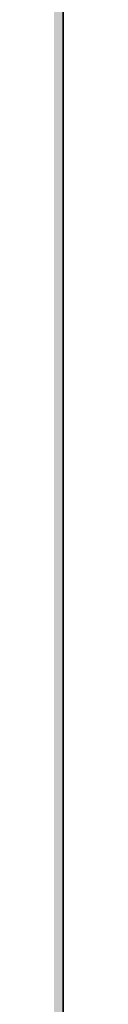
# Model space of a CAD drawing. Units: inches. Extents: x 2083 to 3317, y 1141 to 2115.
# Tile 176 of 256: x 3126.95976 to 3126.95983, y 1263.27402 to 1263.29018. Entities that reach past the tile are written whole.
import ezdxf

# ---------------------------------------------------------------- set-up
doc = ezdxf.new("R2010")
doc.units = ezdxf.units.IN
doc.layers.add('A-ANNO-DIMS', color=2, linetype='Continuous', lineweight=18)
doc.layers.add('A-WALL', color=7, linetype='Continuous', lineweight=35)
doc.layers.add('A-WALL-PATT', color=251, linetype='Continuous', lineweight=13, true_color=0x636466)
doc.styles.get("Standard").update_dxf_attribs({"font": 'arial.ttf'})
doc.dimstyles.new('ISO-25', dxfattribs={"dimtxt": 12, "dimasz": 12, "dimexe": 1.25, "dimexo": 0.625, "dimtad": 1, "dimlunit": 3, "dimtxsty": 'Standard', "dimcen": 2.5, "dimadec": 0, "dimazin": 0, "dimtfac": 1, "dimtmove": 0, "dimatfit": 3, "dimfxl": 1, "dimarcsym": 0})

# ---------------------------------------------------------------- blocks, each defined once
blk = doc.blocks.new('*D9')
at = {"layer": 'A-ANNO-DIMS', "color": 0, "lineweight": -2, "transparency": 16777216}
for p, q in [((3127.584783, 1486.76136), (3190.40309, 1486.76136)), ((3189.15309, 1474.76136), (3189.15309, 1275.26136)), ((3127.584783, 1263.26136), (3190.40309, 1263.26136))]:
    blk.add_line(p, q, dxfattribs=at)
at = {"layer": 'A-ANNO-DIMS', "color": 0, "transparency": 16777216}
for points in [[(3187.15309, 1474.76136), (3191.15309, 1474.76136), (3189.15309, 1486.76136)], [(3187.15309, 1275.26136), (3191.15309, 1275.26136), (3189.15309, 1263.26136)]]:
    blk.add_solid(points, dxfattribs=at)
at = {"layer": 'Defpoints', "color": 0, "transparency": 16777216}
for p in [(3126.959783, 1486.76136), (3126.959783, 1263.26136), (3189.15309, 1263.26136)]:
    blk.add_point(p, dxfattribs=at)
at = {"layer": 'A-ANNO-DIMS', "color": 0, "transparency": 16777216, "insert": (3182.401214, 1375.01136), "char_height": 12, "attachment_point": 5, "rotation": 90}
blk.add_mtext('18\'-7.5"', dxfattribs=at)
blk = doc.blocks.new('*D26')
at = {"layer": 'A-ANNO-DIMS', "color": 0, "lineweight": -2, "transparency": 16777216}
for p, q in [((3088.985844, 1274.915092), (3088.985844, 1270.951963)), ((3111.240037, 1274.915092), (3111.240037, 1270.951963)), ((3076.985844, 1272.201963), (2840.262447, 1272.201963)), ((3111.240037, 1272.201963), (3088.985844, 1272.201963)), ((3123.240037, 1272.201963), (3135.240037, 1272.201963))]:
    blk.add_line(p, q, dxfattribs=at)
at = {"layer": 'A-ANNO-DIMS', "color": 0, "transparency": 16777216}
for points in [[(3076.985844, 1274.201963), (3076.985844, 1270.201963), (3088.985844, 1272.201963)], [(3123.240037, 1274.201963), (3123.240037, 1270.201963), (3111.240037, 1272.201963)]]:
    blk.add_solid(points, dxfattribs=at)
at = {"layer": 'Defpoints', "color": 0, "transparency": 16777216}
for p in [(3088.985844, 1275.540092), (3111.240037, 1275.540092), (3088.985844, 1272.201963)]:
    blk.add_point(p, dxfattribs=at)
at = {"layer": 'A-ANNO-DIMS', "color": 0, "transparency": 16777216, "insert": (2952.624146, 1279.031602), "char_height": 12, "attachment_point": 5}
blk.add_mtext('NIGHTSTAND 1\'-10 1/2" TYP.', dxfattribs=at)
blk = doc.blocks.new('*D27')
at = {"layer": 'A-ANNO-DIMS', "color": 0, "lineweight": -2, "transparency": 16777216}
for p, q in [((3114.578165, 1309.794285), (3114.578165, 1321.794285)), ((3111.865037, 1297.794285), (3115.828165, 1297.794285)), ((3114.578165, 1297.794285), (3114.578165, 1275.540092)), ((3111.865037, 1275.540092), (3115.828165, 1275.540092)), ((3114.578165, 1263.540092), (3114.578165, 1140.988591))]:
    blk.add_line(p, q, dxfattribs=at)
at = {"layer": 'A-ANNO-DIMS', "color": 0, "transparency": 16777216}
for points in [[(3112.578165, 1309.794285), (3116.578165, 1309.794285), (3114.578165, 1297.794285)], [(3112.578165, 1263.540092), (3116.578165, 1263.540092), (3114.578165, 1275.540092)]]:
    blk.add_solid(points, dxfattribs=at)
at = {"layer": 'Defpoints', "color": 0, "transparency": 16777216}
for p in [(3111.240037, 1297.794285), (3111.240037, 1275.540092), (3114.578165, 1275.540092)]:
    blk.add_point(p, dxfattribs=at)
at = {"layer": 'A-ANNO-DIMS', "color": 0, "transparency": 16777216, "insert": (3107.748527, 1196.264342), "char_height": 12, "attachment_point": 5, "rotation": 90}
blk.add_mtext('1\'-10 1/2" TYP.', dxfattribs=at)

msp = doc.modelspace()

# ---------------------------------------------------------------- hatches: boundary and pattern name
at = {"layer": 'A-WALL-PATT'}
h = msp.add_hatch(color=256, dxfattribs=at)
h.dxf.hatch_style = 1
h.paths.add_polyline_path([(3126.959783, 2020.76136), (2748.959783, 2020.76136), (2604.959783, 2020.76136), (2226.959783, 2020.76136), (2226.959783, 1702.76136), (2466.959783, 1702.76136), (2466.959783, 1582.76136), (2418.959783, 1582.76136), (2418.959783, 1477.76136), (2226.959783, 1477.76136), (2226.959783, 1263.26136), (2544.959783, 1263.26136), (2544.959783, 1411.76136), (2604.959783, 1411.76136), (2685.959783, 1411.76136), (2685.959783, 1420.76136), (2604.959783, 1420.76136), (2604.959783, 1573.76136), (2604.959783, 1702.76136), (2604.959783, 2011.76136), (2748.959783, 2011.76136), (2748.959783, 1702.76136), (2862.959783, 1702.76136), (2862.959783, 1621.76136), (2871.959783, 1621.76136), (2871.959783, 1702.76136), (2883.959783, 1702.76136), (2883.959783, 1706.939459, -0.026459), (2883.959783, 1711.76136), (2757.959783, 1711.76136), (2757.959783, 1807.76136), (2787.959783, 1807.76136), (2787.959783, 1812.26136), (2757.959783, 1812.26136), (2757.959783, 2011.76136), (2877.959783, 2011.76136), (2877.959783, 1812.26136), (2847.959783, 1812.26136), (2847.959783, 1807.76136), (2889.835742, 1807.76136), (2889.835742, 1812.26136), (2882.459783, 1812.26136), (2882.459783, 2011.76136), (3117.959783, 2011.76136), (3117.959783, 1812.26136), (2937.835742, 1812.26136), (2937.835742, 1807.76136), (2995.709783, 1807.76136), (2995.709783, 1796.117666), (3000.209783, 1796.117666), (3000.209783, 1807.76136), (3117.959783, 1807.76136), (3117.959783, 1711.76136), (3000.209783, 1711.76136), (3000.209783, 1760.117666), (2998.572705, 1760.117666, -0.020711), (2995.709783, 1760.117666), (2995.709783, 1711.76136), (2931.959783, 1711.76136), (2931.959783, 1702.76136), (3126.959783, 1702.76136)])
h.paths.add_polyline_path([(2471.459783, 2011.76136), (2471.459783, 1810.01136), (2462.716936, 1810.01136), (2462.716936, 1805.51136), (2505.959783, 1805.51136), (2505.959783, 1810.01136), (2475.959783, 1810.01136), (2475.959783, 2011.76136), (2595.959783, 2011.76136), (2595.959783, 1810.01136), (2565.959783, 1810.01136), (2565.959783, 1805.51136), (2595.959783, 1805.51136), (2595.959783, 1711.76136), (2235.959783, 1711.76136), (2235.959783, 1805.51136), (2353.709783, 1805.51136), (2353.709783, 1796.054162), (2358.209783, 1796.054162), (2358.209783, 1805.51136), (2414.716936, 1805.51136), (2414.716936, 1810.01136), (2235.959783, 1810.01136), (2235.959783, 2011.76136)], flags=16)
h.paths.add_polyline_path([(2270.204734, 1994.610008), (2270.204734, 1970.610008), (2246.204734, 1970.610008), (2246.204734, 1994.610008)], flags=0)
edge = h.paths.add_edge_path(flags=0)
edge.add_ellipse((2332.027391, 1899.798176), major_axis=(-3.042994, 3.042994), ratio=0.16825245, start_angle=-161.332166, end_angle=-156.307114, ccw=False)
edge.add_ellipse((2333.082037, 1898.74353), major_axis=(-1.054646, 1.054646), ratio=0.4535321, start_angle=-123.371019, end_angle=-94.159107)
edge = h.paths.add_edge_path(flags=0)
edge.add_ellipse((2332.027391, 1968.87629), major_axis=(3.042994, 3.042994), ratio=0.16825245, start_angle=18.667834, end_angle=23.692886)
edge.add_spline(control_points=[(2332.925596, 1970.691105), (2332.226768, 1970.3361), (2330.893709, 1969.658905), (2328.41308, 1970.932138), (2327.203934, 1967.748712), (2324.709596, 1969.955589), (2322.532822, 1967.012354), (2320.012846, 1971.295812), (2317.680308, 1968.157845), (2316.040526, 1967.102047), (2315.426904, 1966.809602)], knot_values=[0, 0, 0, 0, 2.267059, 4.324559, 6.685584, 8.878641, 11.121502, 14.300359, 17.755284, 19.732645, 19.732645, 19.732645, 19.732645], degree=3, periodic=0)
edge.add_ellipse((2332.027391, 1968.87629), major_axis=(3.042994, 3.042994), ratio=0.16825245, start_angle=18.667834, end_angle=23.692886, ccw=False)
edge.add_ellipse((2333.082037, 1969.930936), major_axis=(1.054646, 1.054646), ratio=0.4535321, start_angle=56.628981, end_angle=85.840893, ccw=False)
edge = h.paths.add_edge_path(flags=0)
edge.add_spline(control_points=[(2296.428287, 1967.987908), (2293.627804, 1965.336314), (2287.703624, 1959.727094), (2299.74386, 1949.995699), (2294.532591, 1935.668528), (2290.573228, 1920.603512), (2293.394124, 1909.973691), (2296.185407, 1904.966543)], knot_values=[0.099185, 0.099185, 0.099185, 0.099185, 0.345301, 0.619822, 0.982653, 1.386093, 1.810555, 1.810555, 1.810555, 1.810555], degree=3, periodic=0)
edge.add_spline(control_points=[(2296.185407, 1904.966543), (2297.383582, 1902.6193), (2298.000969, 1901.949312), (2298.55297, 1901.468155)], knot_values=[0.006246, 0.006246, 0.006246, 0.006246, 0.055476, 0.055476, 0.055476, 0.055476], degree=3, periodic=0)
edge.add_spline(control_points=[(2298.55297, 1901.468155), (2297.258612, 1900.923224), (2295.225294, 1900.232126), (2293.060229, 1900.614205), (2292.101423, 1900.788415), (2292.089578, 1900.790568)], knot_values=[0.312835, 0.312835, 0.312835, 0.312835, 0.40178, 0.474987, 0.475903, 0.475903, 0.475903, 0.475903], degree=3, periodic=0)
edge.add_arc((2292.793646, 1904.664109), 3.937008, 215.420897, 259.698179, ccw=False)
edge.add_spline(control_points=[(2289.585314, 1902.382304), (2289.476652, 1902.535087), (2289.36848, 1902.688035), (2289.260865, 1902.84117)], knot_values=[0.102872, 0.102872, 0.102872, 0.102872, 0.116896, 0.116896, 0.116896, 0.116896], degree=3, periodic=0)
edge.add_spline(control_points=[(2289.260865, 1902.84117), (2288.686604, 1902.550192), (2287.640048, 1902.019902), (2285.881337, 1901.873954), (2283.852972, 1901.504352), (2281.719987, 1899.710538), (2278.466991, 1899.492942), (2276.157136, 1901.883202), (2272.258953, 1899.804071), (2267.777605, 1901.843183), (2262.243882, 1900.184033), (2257.414927, 1901.782061), (2254.318374, 1900.72612), (2253.178285, 1900.337343)], knot_values=[0, 0, 0, 0, 1.907977, 3.477176, 5.261074, 7.972851, 11.680248, 13.717921, 16.939592, 22.789562, 27.502503, 33.595215, 37.145618, 37.145618, 37.145618, 37.145618], degree=3, periodic=0)
edge.add_line((2253.178285, 1900.337343), (2250.24424, 1902.84117))
edge.add_line((2250.24424, 1902.84117), (2250.24424, 1965.833296))
edge.add_line((2250.24424, 1965.833296), (2253.178285, 1968.337123))
edge.add_spline(control_points=[(2253.178285, 1968.337123), (2254.318374, 1967.948346), (2257.414927, 1966.892405), (2262.243882, 1968.490433), (2267.777605, 1966.831283), (2271.52673, 1968.537217), (2273.875914, 1967.828289), (2274.206701, 1967.727642)], knot_values=[0, 0, 0, 0, 0.09018, 0.244935, 0.364644, 0.513233, 0.537855, 0.537855, 0.537855, 0.537855], degree=3, periodic=0)
edge.add_arc((2274.352887, 1963.793349), 3.937008, 72.051134, 92.127949, ccw=False)
edge.add_arc((2281.296933, 1985.230003), 18.596298, 252.0511336, 288.5657217)
edge.add_arc((2292.316717, 1956.02888), 12.646081, 71.0267879, 113.7782184, ccw=False)
edge = h.paths.add_edge_path(flags=0)
edge.add_spline(control_points=[(2274.899415, 1951.856195), (2275.066156, 1951.616592), (2275.232687, 1951.376588), (2275.397987, 1951.135855)], knot_values=[1.409916, 1.409916, 1.409916, 1.409916, 1.43159, 1.43159, 1.43159, 1.43159], degree=3, periodic=0)
edge.add_spline(control_points=[(2275.397987, 1951.135855), (2275.792106, 1950.561885), (2276.179231, 1949.983774), (2276.545546, 1949.397103)], knot_values=[1.358238, 1.358238, 1.358238, 1.358238, 1.409916, 1.409916, 1.409916, 1.409916], degree=3, periodic=0)
edge.add_line((2276.545546, 1949.397103), (2277.437289, 1947.862185))
edge.add_spline(control_points=[(2277.437289, 1947.862185), (2276.303834, 1945.673115), (2274.639698, 1942.426882), (2274.631615, 1938.0939), (2272.799124, 1930.85155), (2274.356426, 1943.897046), (2275.947681, 1947.923356), (2276.545546, 1949.397103)], knot_values=[0.005632, 0.005632, 0.005632, 0.005632, 0.186014, 0.266002, 0.357087, 0.59639, 0.739732, 0.739732, 0.739732, 0.739732], degree=3, periodic=0)
edge.add_spline(control_points=[(2276.545546, 1949.397103), (2276.179231, 1949.983774), (2275.792106, 1950.561885), (2275.397987, 1951.135855)], knot_values=[1.358238, 1.358238, 1.358238, 1.358238, 1.409916, 1.409916, 1.409916, 1.409916], degree=3, periodic=0)
edge.add_spline(control_points=[(2275.397987, 1951.135855), (2274.9425, 1950.080452), (2274.20776, 1948.025272), (2273.934602, 1944.851477), (2272.468534, 1937.627489), (2273.466216, 1945.696466), (2274.700615, 1951.059472), (2274.899415, 1951.856195)], knot_values=[0.104364, 0.104364, 0.104364, 0.104364, 0.189636, 0.269624, 0.36071, 0.600013, 0.644622, 0.644622, 0.644622, 0.644622], degree=3, periodic=0)
h.paths.add_polyline_path([(2269.167514, 1963.127573, -0.357527), (2268.170633, 1960.97637, -0.092561), (2268.170633, 1939.436325, -0.357527), (2269.167514, 1937.285122, -0.357527), (2267.01631, 1938.282002, -0.164785), (2254.685581, 1938.282002, -0.357527), (2252.534378, 1937.285122, -0.357527), (2253.531259, 1939.436325, -0.092561), (2253.531259, 1960.97637, -0.357527), (2252.534378, 1963.127573, -0.357527), (2254.685581, 1962.130692, -0.164785), (2267.01631, 1962.130692, -0.357527)], flags=0)
h.paths.add_polyline_path([(2248.874068, 1967.8018), (2248.874068, 1957.02771), (2249.457783, 1957.02771), (2249.457783, 1911.646756), (2248.874068, 1911.646756), (2248.874068, 1900.872666), (2246.511863, 1900.872666, 0.197327), (2244.149658, 1902.456873), (2244.149658, 1966.217592, 0.197327), (2246.511863, 1967.8018)], flags=0)
h.paths.add_polyline_path([(2269.167514, 1931.389344, -0.357527), (2268.170633, 1929.238141, -0.092561), (2268.170633, 1907.698096, -0.357527), (2269.167514, 1905.546893, -0.357527), (2267.01631, 1906.543774, -0.164785), (2254.685581, 1906.543774, -0.357527), (2252.534378, 1905.546893, -0.357527), (2253.531259, 1907.698096, -0.092561), (2253.531259, 1929.238141, -0.357527), (2252.534378, 1931.389344, -0.357527), (2254.685581, 1930.392463, -0.164785), (2267.01631, 1930.392463, -0.357527)], flags=0)
edge = h.paths.add_edge_path(flags=0)
edge.add_spline(control_points=[(2276.196858, 1906.723702), (2276.168144, 1909.028928), (2276.114049, 1913.371852), (2270.598417, 1924.924978), (2273.905175, 1919.012779), (2275.921711, 1916.262063), (2275.47457, 1912.402149), (2277.257874, 1910.380621), (2276.696044, 1908.225036), (2276.646218, 1906.813023), (2276.617825, 1906.008407)], knot_values=[0, 0, 0, 0, 8.61026, 16.221274, 18.843057, 23.804898, 27.440828, 29.356102, 31.203478, 33.650687, 33.650687, 33.650687, 33.650687], degree=3, periodic=0)
edge.add_spline(control_points=[(2276.617825, 1906.008407), (2276.623313, 1905.624144), (2276.497738, 1904.628661), (2275.441779, 1903.854725), (2274.937314, 1903.08045), (2274.85908, 1902.84117)], knot_values=[0.156488, 0.156488, 0.156488, 0.156488, 0.184398, 0.231376, 0.250598, 0.250598, 0.250598, 0.250598], degree=3, periodic=0)
edge.add_line((2274.85908, 1902.84117), (2276.50598, 1902.84117))
edge.add_spline(control_points=[(2276.50598, 1902.84117), (2276.788308, 1903.08494), (2277.665071, 1904.125196), (2278.249538, 1904.340738), (2277.653872, 1908.527387), (2278.15567, 1906.227808), (2278.100464, 1905.285948), (2278.846675, 1904.069005), (2277.856785, 1903.414948), (2277.874191, 1902.99105), (2277.903562, 1902.84117)], knot_values=[0.059574, 0.059574, 0.059574, 0.059574, 0.080753, 0.103741, 0.16972, 0.176036, 0.207137, 0.240474, 0.262341, 0.27366, 0.27366, 0.27366, 0.27366], degree=3, periodic=0)
edge.add_line((2277.903562, 1902.84117), (2280.029825, 1902.84117))
edge.add_spline(control_points=[(2280.029825, 1902.84117), (2279.888221, 1903.088398), (2279.499257, 1903.981551), (2280.152284, 1905.939349), (2278.103615, 1909.657757), (2279.762395, 1907.185285), (2280.3279, 1904.874861), (2280.485109, 1903.48959), (2281.463269, 1903.249432), (2281.758343, 1902.936497), (2281.834036, 1902.84117)], knot_values=[0.013856, 0.013856, 0.013856, 0.013856, 0.034874, 0.088867, 0.107879, 0.126738, 0.158714, 0.193757, 0.217487, 0.226722, 0.226722, 0.226722, 0.226722], degree=3, periodic=0)
edge.add_spline(control_points=[(2281.834036, 1902.84117), (2281.787535, 1902.826703), (2281.647022, 1902.782988), (2281.395527, 1902.85949), (2281.088077, 1902.985242), (2280.720683, 1903.060902), (2280.333451, 1903.025726), (2280.124767, 1902.898879), (2280.029825, 1902.84117)], knot_values=[0, 0, 0, 0, 0.14413, 0.435517, 0.749276, 1.153046, 1.548371, 1.878348, 1.878348, 1.878348, 1.878348], degree=3, periodic=0)
edge.add_line((2280.029825, 1902.84117), (2277.903562, 1902.84117))
edge.add_spline(control_points=[(2277.903562, 1902.84117), (2277.892855, 1902.795855), (2277.865396, 1902.679637), (2277.607479, 1902.687483), (2277.27405, 1902.8007), (2276.837921, 1902.619775), (2276.583807, 1902.789261), (2276.50598, 1902.84117)], knot_values=[0, 0, 0, 0, 0.127189, 0.326199, 0.628009, 1.24357, 1.515331, 1.515331, 1.515331, 1.515331], degree=3, periodic=0)
edge.add_line((2276.50598, 1902.84117), (2274.85908, 1902.84117))
edge.add_spline(control_points=[(2274.85908, 1902.84117), (2274.814437, 1902.898587), (2274.72513, 1903.013446), (2274.493477, 1903.118968), (2274.244285, 1902.960539), (2273.937121, 1903.184942), (2273.614039, 1902.983143), (2273.408316, 1902.883045), (2273.322254, 1902.84117)], knot_values=[0, 0, 0, 0, 0.21843, 0.436957, 0.687977, 0.990379, 1.398396, 1.69185, 1.69185, 1.69185, 1.69185], degree=3, periodic=0)
edge.add_spline(control_points=[(2273.322254, 1902.84117), (2273.61674, 1903.445692), (2274.273998, 1904.538253), (2276.027239, 1904.573702), (2276.206963, 1906.583637), (2276.196858, 1906.723702)], knot_values=[0.012227, 0.012227, 0.012227, 0.012227, 0.059472, 0.106218, 0.134458, 0.134458, 0.134458, 0.134458], degree=3, periodic=0)
h.paths.add_polyline_path([(2270.776054, 1897.789828), (2270.776054, 1873.789828), (2246.776054, 1873.789828), (2246.776054, 1897.789828)], flags=0)
h.paths.add_polyline_path([(2353.709783, 1760.005059), (2353.709783, 1760.054162), (2358.209783, 1760.054162, -0.033729)], flags=0)
h.paths.add_polyline_path([(2321.819119, 1737.529186), (2341.995327, 1737.529186, -0.414214), (2343.203273, 1736.321241), (2343.203273, 1721.020596, -0.414214), (2341.995327, 1719.812651), (2321.819119, 1719.812651, -0.414214), (2320.611173, 1721.020596), (2320.611173, 1736.321241, -0.414214)], flags=0)
h.paths.add_polyline_path([(2324.23501, 1736.321241), (2339.579436, 1736.321241, -0.414214), (2341.995327, 1733.905349), (2341.995327, 1725.44973, -0.414214), (2339.579436, 1723.033839), (2333.680588, 1723.033839), (2333.845317, 1722.045467, -0.870646), (2335.425399, 1721.825893, -0.767327), (2333.922694, 1721.423245), (2331.291024, 1721.423245, -0.767327), (2329.788319, 1721.825893, -0.870646), (2331.368401, 1722.045467), (2331.53313, 1723.033839), (2324.23501, 1723.033839, -0.414214), (2321.819119, 1725.44973), (2321.819119, 1733.905349, -0.414214)], flags=0)
h.paths.add_polyline_path([(2570.483789, 1928.615444), (2589.683789, 1928.615444), (2590.168829, 1928.615444), (2590.168829, 1904.993397), (2570.483789, 1904.993397)], flags=0)
h.paths.add_polyline_path([(2574.447324, 1927.263822, -1), (2572.828836, 1927.263822, -1)], flags=0)
h.paths.add_polyline_path([(2573.089867, 1926.940877), (2573.925032, 1927.776042), (2574.147743, 1927.553332), (2573.312577, 1926.718166)], flags=0)
h.paths.add_polyline_path([(2578.779065, 1919.729618, -1), (2571.591663, 1919.729618, -1)], flags=0)
h.paths.add_polyline_path([(2578.385364, 1919.729618, -1), (2571.985364, 1919.729618, -1)], flags=0)
h.paths.add_polyline_path([(2331.595764, 1729.476216, -1), (2333.617954, 1729.476216, -1)], flags=0)
h.paths.add_polyline_path([(2578.034228, 1927.263822, -1), (2576.41574, 1927.263822, -1)], flags=0)
h.paths.add_polyline_path([(2576.688851, 1927.531089), (2576.911562, 1927.753799), (2577.746728, 1926.918634), (2577.524017, 1926.695923)], flags=0)
h.paths.add_polyline_path([(2578.139065, 1909.859539, -1), (2572.231663, 1909.859539, -1)], flags=0)
h.paths.add_polyline_path([(2577.745364, 1909.859539, -1), (2572.625364, 1909.859539, -1)], flags=0)
h.paths.add_polyline_path([(2583.797718, 1927.263822, -1), (2582.179229, 1927.263822, -1)], flags=0)
h.paths.add_polyline_path([(2582.718649, 1927.753799), (2583.553814, 1926.918634), (2583.331103, 1926.695923), (2582.495938, 1927.531089)], flags=0)
h.paths.add_polyline_path([(2582.495938, 1927.531089), (2582.718649, 1927.753799), (2583.553814, 1926.918634), (2583.331103, 1926.695923)], flags=0)
h.paths.add_polyline_path([(2587.739065, 1920.529618, -1), (2581.831663, 1920.529618, -1)], flags=0)
h.paths.add_polyline_path([(2587.345364, 1920.529618, -1), (2582.225364, 1920.529618, -1)], flags=0)
h.paths.add_polyline_path([(2587.384622, 1927.263822, -1), (2585.766133, 1927.263822, -1)], flags=0)
h.paths.add_polyline_path([(2586.081993, 1926.980247), (2586.917158, 1927.815412), (2587.139869, 1927.592702), (2586.304703, 1926.757536)], flags=0)
h.paths.add_polyline_path([(2588.379065, 1910.659539, -1), (2581.191663, 1910.659539, -1)], flags=0)
h.paths.add_polyline_path([(2587.985364, 1910.659539, -1), (2581.585364, 1910.659539, -1)], flags=0)
h.paths.add_polyline_path([(2417.167729, 1729.477895), (2437.343937, 1729.477895, -0.414214), (2438.551883, 1728.26995), (2438.551883, 1712.969306, -0.414214), (2437.343937, 1711.76136), (2417.167729, 1711.76136, -0.414214), (2415.959783, 1712.969306), (2415.959783, 1728.26995, -0.414214)], flags=0)
h.paths.add_polyline_path([(2419.58362, 1728.26995), (2434.928046, 1728.26995, -0.414214), (2437.343937, 1725.854059), (2437.343937, 1717.39844, -0.414214), (2434.928046, 1714.982548), (2429.029199, 1714.982548), (2429.193927, 1713.994176, -0.870646), (2430.774009, 1713.774603, -0.767327), (2429.271304, 1713.371954), (2426.639634, 1713.371954, -0.767327), (2425.136929, 1713.774603, -0.870646), (2426.717011, 1713.994176), (2426.88174, 1714.982548), (2419.58362, 1714.982548, -0.414214), (2417.167729, 1717.39844), (2417.167729, 1725.854059, -0.414214)], flags=0)
h.paths.add_polyline_path([(2419.58362, 1728.26995), (2434.928046, 1728.26995, -0.414214), (2437.343937, 1725.854059), (2437.343937, 1717.39844, -0.414214), (2434.928046, 1714.982548), (2429.029199, 1714.982548), (2428.358118, 1719.009034), (2427.552821, 1719.009034), (2426.88174, 1714.982548), (2419.58362, 1714.982548, -0.414214), (2417.167729, 1717.39844), (2417.167729, 1725.854059, -0.414214)], flags=0)
h.paths.add_polyline_path([(2426.944374, 1721.424925, -1), (2428.966564, 1721.424925, -1)], flags=0)
h.paths.add_polyline_path([(2475.959783, 1702.76136), (2595.959783, 1702.76136), (2595.959783, 1582.76136), (2475.959783, 1582.76136)], flags=16)
h.paths.add_polyline_path([(2427.959783, 1573.76136), (2595.959783, 1573.76136), (2595.959783, 1468.76136), (2595.959783, 1420.76136), (2384.459783, 1420.76136), (2384.459783, 1468.76136), (2427.959783, 1468.76136)], flags=16)
h.paths.add_polyline_path([(2379.959783, 1468.76136), (2379.959783, 1420.76136), (2235.959783, 1420.76136), (2235.959783, 1468.76136)], flags=16)
h.paths.add_polyline_path([(2317.815996, 1466.695767), (2337.992205, 1466.695767, -0.414214), (2339.20015, 1465.487821), (2339.20015, 1450.187177, -0.414214), (2337.992205, 1448.979232), (2317.815996, 1448.979232, -0.414214), (2316.608051, 1450.187177), (2316.608051, 1465.487821, -0.414214)], flags=0)
h.paths.add_polyline_path([(2320.231887, 1465.487821), (2335.576313, 1465.487821, -0.414214), (2337.992205, 1463.07193), (2337.992205, 1454.616311, -0.414214), (2335.576313, 1452.20042), (2329.677466, 1452.20042), (2329.842195, 1451.212047, -0.870646), (2331.422276, 1450.992474, -0.767327), (2329.919571, 1450.589826), (2327.287902, 1450.589826, -0.767327), (2325.785197, 1450.992474, -0.870646), (2327.365278, 1451.212047), (2327.530007, 1452.20042), (2320.231887, 1452.20042, -0.414214), (2317.815996, 1454.616311), (2317.815996, 1463.07193, -0.414214)], flags=0)
h.paths.add_polyline_path([(2320.231887, 1465.487821), (2335.576313, 1465.487821, -0.414214), (2337.992205, 1463.07193), (2337.992205, 1454.616311, -0.414214), (2335.576313, 1452.20042), (2329.677466, 1452.20042), (2329.006385, 1456.226905), (2328.201088, 1456.226905), (2327.530007, 1452.20042), (2320.231887, 1452.20042, -0.414214), (2317.815996, 1454.616311), (2317.815996, 1463.07193, -0.414214)], flags=0)
h.paths.add_polyline_path([(2327.592641, 1458.642796, -1), (2329.614832, 1458.642796, -1)], flags=0)
h.paths.add_polyline_path([(2244.411744, 1433.340453), (2241.920945, 1433.340453, -0.414214), (2240.017856, 1435.243542), (2240.017856, 1440.952808, -0.414211), (2241.920925, 1442.855897), (2244.411744, 1442.855897, -1.976472)], flags=0)
h.paths.add_polyline_path([(2245.356888, 1434.397536, -0.414214), (2245.356888, 1441.798814, -2.144098)], flags=0)
h.paths.add_polyline_path([(2535.959783, 1416.26136), (2535.959783, 1272.26136), (2235.959783, 1272.26136), (2235.959783, 1416.26136)], flags=16)
h.paths.add_polyline_path([(2260.119561, 1384.292841), (2260.119561, 1362.038649), (2237.865369, 1362.038649), (2237.865369, 1384.292841)], flags=0)
edge = h.paths.add_edge_path(flags=0)
edge.add_line((2318.251847, 1362.093298), (2318.145797, 1362.000973))
edge.add_ellipse((2317.445116, 1360.431044), major_axis=(2.82164, 2.82164), ratio=0.16825245, start_angle=18.667834, end_angle=20.948127, ccw=False)
edge.add_ellipse((2318.423045, 1361.408974), major_axis=(0.977929, 0.977929), ratio=0.4535321, start_angle=56.628981, end_angle=70.226201, ccw=False)
edge = h.paths.add_edge_path(flags=0)
edge.add_line((2319.10737, 1295.571078), (2319.015044, 1295.677128))
edge.add_ellipse((2317.445116, 1296.377809), major_axis=(-2.82164, 2.82164), ratio=0.16825245, start_angle=-161.332166, end_angle=-159.051873, ccw=False)
edge.add_ellipse((2318.423045, 1295.39988), major_axis=(-0.977929, 0.977929), ratio=0.4535321, start_angle=-123.371019, end_angle=-109.773799)
edge = h.paths.add_edge_path(flags=0)
edge.add_spline(control_points=[(2284.210349, 1301.170219), (2284.580688, 1300.444719), (2284.891189, 1299.892024), (2285.159553, 1299.461018)], knot_values=[0.039066, 0.039066, 0.039066, 0.039066, 0.055476, 0.055476, 0.055476, 0.055476], degree=3, periodic=0)
edge.add_line((2285.159553, 1299.461018), (2284.210349, 1301.170219))
edge = h.paths.add_edge_path(flags=0)
edge.add_line((2280.412458, 1297.298013), (2283.369991, 1297.036122))
edge.add_line((2283.369991, 1297.036122), (2286.40569, 1297.92631))
edge.add_spline(control_points=[(2286.40569, 1297.92631), (2285.305487, 1297.463119), (2284.344777, 1297.129151), (2283.369991, 1297.036122)], knot_values=[0.394369, 0.394369, 0.394369, 0.394369, 0.475903, 0.475903, 0.475903, 0.475903], degree=3, periodic=0)
edge.add_spline(control_points=[(2283.369991, 1297.036122), (2283.28139, 1297.027666), (2282.316289, 1296.957336), (2281.312502, 1297.134479), (2280.423441, 1297.296016), (2280.412458, 1297.298013)], knot_values=[0.312835, 0.312835, 0.312835, 0.312835, 0.320246, 0.393453, 0.394369, 0.394369, 0.394369, 0.394369], degree=3, periodic=0)
edge = h.paths.add_edge_path(flags=0)
edge.add_line((2284.435561, 1359.607285), (2280.446291, 1355.328047))
edge.add_line((2280.446291, 1355.328047), (2279.579987, 1351.017754))
edge.add_line((2279.579987, 1351.017754), (2282.412974, 1346.580433))
edge.add_spline(control_points=[(2282.412974, 1346.580433), (2283.153331, 1345.589236), (2284.252896, 1344.028897), (2284.801037, 1342.387167), (2284.935162, 1341.805544)], knot_values=[1.240098, 1.240098, 1.240098, 1.240098, 1.332892, 1.382712, 1.382712, 1.382712, 1.382712], degree=3, periodic=0)
edge.add_spline(control_points=[(2284.935162, 1341.805544), (2285.319108, 1340.1406), (2285.233029, 1338.409204), (2284.909938, 1336.654122)], knot_values=[1.097484, 1.097484, 1.097484, 1.097484, 1.240098, 1.240098, 1.240098, 1.240098], degree=3, periodic=0)
edge.add_spline(control_points=[(2284.909938, 1336.654122), (2284.586848, 1334.89904), (2284.026745, 1333.120272), (2283.462644, 1331.360585)], knot_values=[0.95487, 0.95487, 0.95487, 0.95487, 1.097484, 1.097484, 1.097484, 1.097484], degree=3, periodic=0)
edge.add_line((2283.462644, 1331.360585), (2281.890376, 1326.153357))
edge.add_line((2281.890376, 1326.153357), (2280.756259, 1321.056089))
edge.add_line((2280.756259, 1321.056089), (2280.299205, 1316.001977))
edge.add_line((2280.299205, 1316.001977), (2280.715933, 1310.950068))
edge.add_line((2280.715933, 1310.950068), (2282.028094, 1305.972137))
edge.add_line((2282.028094, 1305.972137), (2284.210349, 1301.170219))
edge.add_spline(control_points=[(2284.210349, 1301.170219), (2283.340731, 1302.730185), (2282.611904, 1304.336493), (2282.028094, 1305.972137)], knot_values=[0.099185, 0.099185, 0.099185, 0.099185, 0.241799, 0.241799, 0.241799, 0.241799], degree=3, periodic=0)
edge.add_spline(control_points=[(2282.028094, 1305.972137), (2281.444283, 1307.60778), (2281.005489, 1309.272759), (2280.715933, 1310.950068)], knot_values=[0.241799, 0.241799, 0.241799, 0.241799, 0.384413, 0.384413, 0.384413, 0.384413], degree=3, periodic=0)
edge.add_spline(control_points=[(2280.715933, 1310.950068), (2280.433241, 1312.587613), (2280.289386, 1314.276959), (2280.298894, 1315.962032), (2280.299205, 1316.001977)], knot_values=[0.384413, 0.384413, 0.384413, 0.384413, 0.523647, 0.527028, 0.527028, 0.527028, 0.527028], degree=3, periodic=0)
edge.add_spline(control_points=[(2280.299205, 1316.001977), (2280.312326, 1317.686955), (2280.477871, 1319.367926), (2280.756259, 1321.056089)], knot_values=[0.527028, 0.527028, 0.527028, 0.527028, 0.669642, 0.669642, 0.669642, 0.669642], degree=3, periodic=0)
edge.add_spline(control_points=[(2280.756259, 1321.056089), (2281.034648, 1322.744252), (2281.42588, 1324.439608), (2281.890376, 1326.153357)], knot_values=[0.669642, 0.669642, 0.669642, 0.669642, 0.812256, 0.812256, 0.812256, 0.812256], degree=3, periodic=0)
edge.add_spline(control_points=[(2281.890376, 1326.153357), (2282.264383, 1327.533251), (2282.78787, 1329.26181), (2283.352751, 1331.01778), (2283.462644, 1331.360585)], knot_values=[0.812256, 0.812256, 0.812256, 0.812256, 0.927087, 0.95487, 0.95487, 0.95487, 0.95487], degree=3, periodic=0)
edge.add_line((2283.462644, 1331.360585), (2284.909938, 1336.654122))
edge.add_line((2284.909938, 1336.654122), (2284.935162, 1341.805544))
edge.add_line((2284.935162, 1341.805544), (2282.412974, 1346.580433))
edge.add_spline(control_points=[(2282.412974, 1346.580433), (2281.275127, 1348.103792), (2280.078447, 1349.570318), (2279.579987, 1351.017754)], knot_values=[1.382712, 1.382712, 1.382712, 1.382712, 1.525326, 1.525326, 1.525326, 1.525326], degree=3, periodic=0)
edge.add_spline(control_points=[(2279.579987, 1351.017754), (2279.443282, 1351.414721), (2279.136312, 1352.856922), (2279.73519, 1354.290385), (2280.446291, 1355.328047)], knot_values=[1.525326, 1.525326, 1.525326, 1.525326, 1.564439, 1.667941, 1.667941, 1.667941, 1.667941], degree=3, periodic=0)
edge.add_spline(control_points=[(2280.446291, 1355.328047), (2281.426113, 1356.757835), (2282.930837, 1358.18256), (2284.435561, 1359.607285)], knot_values=[1.667941, 1.667941, 1.667941, 1.667941, 1.810555, 1.810555, 1.810555, 1.810555], degree=3, periodic=0)
edge.add_arc((2280.623075, 1348.518181), 11.72618, 71.0267879, 113.7782184)
edge.add_arc((2270.404892, 1375.595156), 17.243567, 252.0511336, 288.5657217, ccw=False)
edge.add_arc((2263.965969, 1355.717847), 3.650622, 72.051134, 92.127949)
edge.add_arc((2263.965969, 1355.717847), 3.650622, 92.127949, 177.98513)
edge.add_spline(control_points=[(2260.317604, 1355.846199), (2260.260417, 1354.220668), (2260.551278, 1350.186547), (2262.999344, 1346.766251), (2264.472741, 1344.649024)], knot_values=[1.43159, 1.43159, 1.43159, 1.43159, 1.564144, 1.770695, 1.770695, 1.770695, 1.770695], degree=3, periodic=0)
edge.add_line((2264.472741, 1344.649024), (2264.93559, 1343.98253))
edge.add_spline(control_points=[(2263.801044, 1340.248105), (2263.843238, 1340.514088), (2264.067244, 1341.756465), (2264.512693, 1343.002453), (2264.935047, 1343.981083)], knot_values=[0.53657, 0.53657, 0.53657, 0.53657, 0.559349, 0.644622, 0.644622, 0.644622, 0.644622], degree=3, periodic=0)
edge.add_spline(control_points=[(2264.935047, 1343.981083), (2265.117771, 1343.714975), (2265.298875, 1343.447906), (2265.476756, 1343.179365)], knot_values=[1.384077, 1.384077, 1.384077, 1.384077, 1.409916, 1.409916, 1.409916, 1.409916], degree=3, periodic=0)
edge.add_spline(control_points=[(2265.476756, 1343.179365), (2265.654637, 1342.910823), (2265.829296, 1342.64081), (2265.99913, 1342.368812)], knot_values=[1.358238, 1.358238, 1.358238, 1.358238, 1.384077, 1.384077, 1.384077, 1.384077], degree=3, periodic=0)
edge.add_line((2265.99913, 1342.368812), (2266.826006, 1340.945547))
edge.add_spline(control_points=[(2266.826006, 1340.945547), (2268.894401, 1337.089691), (2271.398173, 1325.843001), (2270.516164, 1310.568557), (2275.919376, 1301.860609), (2277.789511, 1299.19945)], knot_values=[0.116896, 0.116896, 0.116896, 0.116896, 0.472987, 1.050969, 1.313793, 1.313793, 1.313793, 1.313793], degree=3, periodic=0)
edge.add_spline(control_points=[(2277.789511, 1299.19945), (2277.839405, 1299.128452), (2277.889428, 1299.057498), (2277.939572, 1298.986584)], knot_values=[0.109884, 0.109884, 0.109884, 0.109884, 0.116896, 0.116896, 0.116896, 0.116896], degree=3, periodic=0)
edge.add_line((2277.939572, 1298.986584), (2277.788849, 1299.199114))
edge.add_spline(control_points=[(2277.788849, 1299.199114), (2277.256582, 1298.929414), (2276.28635, 1298.437902), (2275.039352, 1298.334419), (2274.38333, 1298.238895), (2274.215254, 1298.209338)], knot_values=[33.12187, 33.12187, 33.12187, 33.12187, 35.029056, 36.598255, 37.144827, 37.144827, 37.144827, 37.144827], degree=3, periodic=0)
edge.add_line((2274.215254, 1298.209338), (2273.073147, 1297.892961))
edge.add_spline(control_points=[(2273.073147, 1297.892961), (2272.322936, 1297.579784), (2271.039151, 1296.510508), (2269.248395, 1296.226062), (2268.4231, 1296.374654)], knot_values=[26.532584, 26.532584, 26.532584, 26.532584, 29.198919, 31.839101, 31.839101, 31.839101, 31.839101], degree=3, periodic=0)
edge.add_line((2268.4231, 1296.374654), (2263.878501, 1297.457534))
edge.add_spline(control_points=[(2263.878501, 1297.457534), (2263.556077, 1297.359435), (2261.860306, 1296.838694), (2260.23878, 1297.282407), (2258.933454, 1297.516461)], knot_values=[15.919551, 15.919551, 15.919551, 15.919551, 16.939592, 21.226067, 21.226067, 21.226067, 21.226067], degree=3, periodic=0)
edge.add_line((2258.933454, 1297.516461), (2254.055233, 1297.32901))
edge.add_spline(control_points=[(2254.055233, 1297.32901), (2253.755525, 1297.295815), (2252.113683, 1297.165174), (2250.461869, 1297.544221), (2249.129686, 1297.667882)], knot_values=[5.306517, 5.306517, 5.306517, 5.306517, 6.276435, 10.613034, 10.613034, 10.613034, 10.613034], degree=3, periodic=0)
edge.add_line((2249.129686, 1297.667882), (2244.33165, 1296.877756))
edge.add_line((2244.33165, 1296.877756), (2241.611033, 1299.19945))
edge.add_line((2241.611033, 1299.19945), (2241.611033, 1357.609404))
edge.add_line((2241.611033, 1357.609404), (2244.33165, 1359.931097))
edge.add_line((2244.33165, 1359.931097), (2252.728823, 1359.542692))
edge.add_spline(control_points=[(2252.728823, 1359.542692), (2252.870939, 1359.54644), (2253.30574, 1359.548172), (2253.739845, 1359.514274), (2254.031742, 1359.482426)], knot_values=[0.233291, 0.233291, 0.233291, 0.233291, 0.244935, 0.268927, 0.268927, 0.268927, 0.268927], degree=3, periodic=0)
edge.add_line((2254.031742, 1359.482426), (2259.58719, 1359.41639))
edge.add_spline(control_points=[(2259.58719, 1359.41639), (2260.677068, 1359.628503), (2262.073197, 1359.897003), (2263.523692, 1359.459278), (2263.830417, 1359.365952)], knot_values=[0.422516, 0.422516, 0.422516, 0.422516, 0.513233, 0.537855, 0.537855, 0.537855, 0.537855], degree=3, periodic=0)
edge.add_arc((2263.965969, 1355.717847), 3.650622, 72.051134, 92.127949, ccw=False)
edge.add_arc((2270.404892, 1375.595156), 17.243567, 252.0511336, 288.5657217)
edge.add_arc((2280.623075, 1348.518181), 11.72618, 71.0267879, 113.7782184, ccw=False)
h.paths.add_polyline_path([(2240.34053, 1359.434715), (2240.34053, 1349.444353), (2240.881785, 1349.444353), (2240.881785, 1307.3645), (2240.34053, 1307.3645), (2240.34053, 1297.374138), (2238.150157, 1297.374138, 0.197327), (2235.959783, 1298.843108), (2235.959783, 1357.965746, 0.197327), (2238.150157, 1359.434715)], flags=0)
h.paths.add_polyline_path([(2259.15779, 1355.1005, -0.357527), (2258.233425, 1353.10578, -0.092561), (2258.233425, 1333.132601, -0.357527), (2259.15779, 1331.13788, -0.357527), (2257.16307, 1332.062246, -0.164785), (2245.729302, 1332.062246, -0.357527), (2243.734582, 1331.13788, -0.357527), (2244.658947, 1333.132601, -0.092561), (2244.658947, 1353.10578, -0.357527), (2243.734582, 1355.1005, -0.357527), (2245.729302, 1354.176135, -0.164785), (2257.16307, 1354.176135, -0.357527)], flags=0)
edge = h.paths.add_edge_path(flags=0)
edge.add_line((2265.99913, 1342.368812), (2266.826006, 1340.945547))
edge.add_line((2266.826006, 1340.945547), (2265.307557, 1337.814066))
edge.add_line((2265.307557, 1337.814066), (2264.358232, 1334.652939))
edge.add_line((2264.358232, 1334.652939), (2264.262012, 1333.799705))
edge.add_spline(control_points=[(2264.262012, 1333.799705), (2264.208357, 1333.187055), (2264.16206, 1332.365525), (2264.007144, 1331.413933), (2263.969049, 1331.201834)], knot_values=[0.464444, 0.464444, 0.464444, 0.464444, 0.516691, 0.531608, 0.531608, 0.531608, 0.531608], degree=3, periodic=0)
edge.add_spline(control_points=[(2263.969049, 1331.201834), (2263.774535, 1330.118873), (2263.42437, 1328.790839), (2263.25742, 1328.530652), (2263.234028, 1328.514612)], knot_values=[0.372682, 0.372682, 0.372682, 0.372682, 0.44885, 0.464444, 0.464444, 0.464444, 0.464444], degree=3, periodic=0)
edge.add_spline(control_points=[(2263.234028, 1328.514612), (2263.096382, 1328.420227), (2263.13117, 1329.301477), (2263.274953, 1330.615749)], knot_values=[0.280919, 0.280919, 0.280919, 0.280919, 0.372682, 0.372682, 0.372682, 0.372682], degree=3, periodic=0)
edge.add_spline(control_points=[(2263.274953, 1330.615749), (2263.418736, 1331.930022), (2263.671515, 1333.677318), (2263.969852, 1335.315027)], knot_values=[0.189157, 0.189157, 0.189157, 0.189157, 0.280919, 0.280919, 0.280919, 0.280919], degree=3, periodic=0)
edge.add_spline(control_points=[(2263.969852, 1335.315027), (2264.100496, 1336.032192), (2264.418783, 1337.621911), (2264.754848, 1338.86443), (2264.947419, 1339.491124)], knot_values=[0.097394, 0.097394, 0.097394, 0.097394, 0.137578, 0.189157, 0.189157, 0.189157, 0.189157], degree=3, periodic=0)
edge.add_spline(control_points=[(2264.947419, 1339.491124), (2265.290017, 1340.606055), (2265.644238, 1341.493996), (2265.99913, 1342.368812)], knot_values=[0.005632, 0.005632, 0.005632, 0.005632, 0.097394, 0.097394, 0.097394, 0.097394], degree=3, periodic=0)
h.paths.add_polyline_path([(2259.15779, 1325.670973, -0.357527), (2258.233425, 1323.676253, -0.092561), (2258.233425, 1303.703073, -0.357527), (2259.15779, 1301.708353, -0.357527), (2257.16307, 1302.632719, -0.164785), (2245.729302, 1302.632719, -0.357527), (2243.734582, 1301.708353, -0.357527), (2244.658947, 1303.703073, -0.092561), (2244.658947, 1323.676253, -0.357527), (2243.734582, 1325.670973, -0.357527), (2245.729302, 1324.746608, -0.164785), (2257.16307, 1324.746608, -0.357527)], flags=0)
edge = h.paths.add_edge_path(flags=0)
edge.add_spline(control_points=[(2261.708938, 1317.311421), (2261.679482, 1317.41758), (2261.761858, 1317.388535), (2262.490736, 1316.089873), (2262.962185, 1315.300897)], knot_values=[14.955861, 14.955861, 14.955861, 14.955861, 16.221274, 18.694826, 18.694826, 18.694826, 18.694826], degree=3, periodic=0)
edge.add_spline(control_points=[(2262.962185, 1315.300897), (2262.990437, 1315.253617), (2263.702096, 1314.067376), (2264.348983, 1313.127153), (2264.730054, 1312.164154)], knot_values=[18.694826, 18.694826, 18.694826, 18.694826, 18.843057, 22.433791, 22.433791, 22.433791, 22.433791], degree=3, periodic=0)
edge.add_spline(control_points=[(2264.730054, 1312.164154), (2264.875565, 1311.796437), (2265.176873, 1310.769807), (2265.143069, 1309.559262), (2265.247736, 1308.824193)], knot_values=[22.433791, 22.433791, 22.433791, 22.433791, 23.804898, 26.172756, 26.172756, 26.172756, 26.172756], degree=3, periodic=0)
edge.add_line((2265.247736, 1308.824193), (2265.850774, 1307.171888))
edge.add_spline(control_points=[(2265.850774, 1307.171888), (2266.065025, 1306.821678), (2266.384387, 1306.332246), (2266.4244, 1305.780549), (2266.420369, 1305.611216)], knot_values=[28.062562, 28.062562, 28.062562, 28.062562, 29.356102, 29.911721, 29.911721, 29.911721, 29.911721], degree=3, periodic=0)
edge.add_spline(control_points=[(2266.420369, 1305.611216), (2266.416116, 1305.43259), (2266.393999, 1305.249998), (2266.364777, 1305.065857)], knot_values=[29.911721, 29.911721, 29.911721, 29.911721, 30.497837, 30.497837, 30.497837, 30.497837], degree=3, periodic=0)
edge.add_line((2266.364777, 1305.065857), (2266.066151, 1302.136295))
edge.add_spline(control_points=[(2266.066151, 1302.136295), (2266.07124, 1301.779984), (2265.998076, 1301.199985), (2265.663266, 1300.758961), (2265.508908, 1300.585882)], knot_values=[0.156488, 0.156488, 0.156488, 0.156488, 0.184398, 0.203543, 0.203543, 0.203543, 0.203543], degree=3, periodic=0)
edge.add_line((2265.508908, 1300.585882), (2264.435341, 1299.19945))
edge.add_line((2264.435341, 1299.19945), (2265.962442, 1299.19945))
edge.add_line((2265.962442, 1299.19945), (2267.33599, 1301.175276))
edge.add_line((2267.33599, 1301.175276), (2267.311667, 1301.986237))
edge.add_spline(control_points=[(2267.311667, 1301.986237), (2267.261111, 1302.862396), (2267.160212, 1303.737132), (2267.271486, 1303.325896)], knot_values=[0.126229, 0.126229, 0.126229, 0.126229, 0.166617, 0.166617, 0.166617, 0.166617], degree=3, periodic=0)
edge.add_spline(control_points=[(2267.271486, 1303.325896), (2267.280035, 1303.294305), (2267.309785, 1303.175366), (2267.37345, 1302.883608), (2267.406123, 1302.682829), (2267.417926, 1302.601025)], knot_values=[0.166617, 0.166617, 0.166617, 0.166617, 0.16972, 0.176036, 0.180765, 0.180765, 0.180765, 0.180765], degree=3, periodic=0)
edge.add_spline(control_points=[(2267.743891, 1300.987505), (2267.687583, 1301.150943), (2267.48052, 1301.656664), (2267.483751, 1302.144788), (2267.417926, 1302.601025)], knot_values=[0.180765, 0.180765, 0.180765, 0.180765, 0.193767, 0.220139, 0.220139, 0.220139, 0.220139], degree=3, periodic=0)
edge.add_line((2267.417926, 1302.601025), (2267.743891, 1300.987505))
edge.add_spline(control_points=[(2267.743891, 1300.987505), (2267.831961, 1300.731878), (2267.932021, 1300.309904), (2267.554841, 1299.974518), (2267.429366, 1299.829207)], knot_values=[0.220139, 0.220139, 0.220139, 0.220139, 0.240474, 0.25489, 0.25489, 0.25489, 0.25489], degree=3, periodic=0)
edge.add_line((2267.429366, 1299.829207), (2267.258361, 1299.19945))
edge.add_line((2267.258361, 1299.19945), (2269.229956, 1299.19945))
edge.add_spline(control_points=[(2269.229956, 1299.19945), (2269.098653, 1299.428694), (2268.842774, 1300.016251), (2269.011575, 1300.915923), (2268.946796, 1301.66074)], knot_values=[0.013856, 0.013856, 0.013856, 0.013856, 0.034874, 0.067073, 0.067073, 0.067073, 0.067073], degree=3, periodic=0)
edge.add_line((2268.946796, 1301.66074), (2268.431582, 1303.603109))
edge.add_spline(control_points=[(2268.431582, 1303.603109), (2268.175596, 1304.192375), (2267.596214, 1305.251298), (2268.040698, 1304.62321), (2268.251394, 1304.282421)], knot_values=[0.090155, 0.090155, 0.090155, 0.090155, 0.107879, 0.120289, 0.120289, 0.120289, 0.120289], degree=3, periodic=0)
edge.add_spline(control_points=[(2268.251394, 1304.282421), (2268.360882, 1304.105329), (2269.057753, 1302.917983), (2269.382691, 1301.590419), (2269.521405, 1300.775931), (2269.57522, 1300.555784)], knot_values=[0.120289, 0.120289, 0.120289, 0.120289, 0.126738, 0.158714, 0.173506, 0.173506, 0.173506, 0.173506], degree=3, periodic=0)
edge.add_line((2269.57522, 1300.555784), (2270.685798, 1299.421258))
edge.add_spline(control_points=[(2270.685798, 1299.421258), (2270.767221, 1299.357251), (2270.837852, 1299.281401), (2270.902925, 1299.19945)], knot_values=[0.21816, 0.21816, 0.21816, 0.21816, 0.226722, 0.226722, 0.226722, 0.226722], degree=3, periodic=0)
edge.add_line((2270.937201, 1299.192913), (2270.902925, 1299.19945))
edge.add_spline(control_points=[(2270.902925, 1299.19945), (2270.859806, 1299.186035), (2270.729515, 1299.1455), (2270.496314, 1299.216437), (2270.271661, 1299.308323), (2270.121017, 1299.347961), (2270.063339, 1299.359557)], knot_values=[0.939174, 0.939174, 0.939174, 0.939174, 1.083304, 1.374691, 1.68845, 1.878348, 1.878348, 1.878348, 1.878348], degree=3, periodic=0)
edge.add_line((2270.063339, 1299.359557), (2269.229956, 1299.19945))
edge.add_line((2269.229956, 1299.19945), (2267.258361, 1299.19945))
edge.add_spline(control_points=[(2267.258361, 1299.19945), (2267.248433, 1299.157431), (2267.222971, 1299.049667), (2266.983816, 1299.056942), (2266.80921, 1299.11623), (2266.676905, 1299.109091), (2266.636531, 1299.104815)], knot_values=[0.757665, 0.757665, 0.757665, 0.757665, 0.884854, 1.083864, 1.385675, 1.515331, 1.515331, 1.515331, 1.515331], degree=3, periodic=0)
edge.add_spline(control_points=[(2266.636531, 1299.104815), (2266.485225, 1299.088788), (2266.235807, 1299.017123), (2266.034608, 1299.151317), (2265.962442, 1299.19945)], knot_values=[0, 0, 0, 0, 0.485905, 0.757665, 0.757665, 0.757665, 0.757665], degree=3, periodic=0)
edge.add_line((2265.962442, 1299.19945), (2264.435341, 1299.19945))
edge.add_line((2264.435341, 1299.19945), (2263.858444, 1299.367118))
edge.add_spline(control_points=[(2263.858444, 1299.367118), (2263.818943, 1299.370905), (2263.779528, 1299.385721), (2263.740131, 1299.401504)], knot_values=[0.845925, 0.845925, 0.845925, 0.845925, 0.978627, 0.978627, 0.978627, 0.978627], degree=3, periodic=0)
edge.add_line((2263.721786, 1299.396425), (2263.010306, 1299.19945))
edge.add_spline(control_points=[(2263.010306, 1299.19945), (2263.245794, 1299.682859), (2263.506032, 1300.128107), (2263.873494, 1300.408028)], knot_values=[0.012227, 0.012227, 0.012227, 0.012227, 0.052971, 0.052971, 0.052971, 0.052971], degree=3, periodic=0)
edge.add_spline(control_points=[(2263.873494, 1300.408028), (2263.932131, 1300.452695), (2264.084243, 1300.552979), (2264.255189, 1300.624223), (2264.359686, 1300.664747)], knot_values=[0.052971, 0.052971, 0.052971, 0.052971, 0.059472, 0.069086, 0.069086, 0.069086, 0.069086], degree=3, periodic=0)
edge.add_line((2264.359686, 1300.664747), (2265.1419, 1301.077774))
edge.add_line((2265.1419, 1301.077774), (2265.675806, 1302.799558))
edge.add_line((2265.675806, 1302.799558), (2265.5407, 1305.704066))
edge.add_line((2265.5407, 1305.704066), (2264.803073, 1309.327724))
edge.add_line((2264.803073, 1309.327724), (2263.040535, 1314.091791))
edge.add_spline(control_points=[(2263.040535, 1314.091791), (2262.383572, 1315.671438), (2261.795972, 1316.997749), (2261.708938, 1317.311421)], knot_values=[11.216896, 11.216896, 11.216896, 11.216896, 14.955861, 14.955861, 14.955861, 14.955861], degree=3, periodic=0)
h.paths.add_polyline_path([(2871.959783, 1416.26136), (2895.910047, 1416.26136), (2895.910047, 1420.76136), (2871.959783, 1420.76136), (2871.959783, 1501.76136), (2862.959783, 1501.76136), (2862.959783, 1420.76136), (2805.959783, 1420.76136), (2805.959783, 1411.76136), (2862.959783, 1411.76136), (2862.959783, 1263.26136), (3126.959783, 1263.26136), (3126.959783, 1411.76136), (3126.959783, 1486.76136), (2943.959783, 1486.76136), (2943.959783, 1477.76136), (2967.860311, 1477.76136), (2967.860311, 1420.76136), (2943.910047, 1420.76136), (2943.910047, 1416.26136), (3117.959783, 1416.26136), (3117.959783, 1420.76136), (2972.360311, 1420.76136), (2972.360311, 1477.76136), (3117.959783, 1477.76136), (3117.959783, 1420.76136), (3117.959783, 1272.26136), (2871.959783, 1272.26136)], flags=0)
h.paths.add_polyline_path([(2457.125626, 1485.942505), (2527.602651, 1485.942505), (2527.602651, 1537.635702), (2457.125626, 1537.635702)], flags=8)
h.paths.add_polyline_path([(2481.005058, 1609.981804), (2590.765818, 1609.981804), (2590.765818, 1682.003362), (2481.005058, 1682.003362)], flags=8)
h.paths.add_polyline_path([(2483.085022, 1729.126784), (2553.562048, 1729.126784), (2553.562048, 1780.81998), (2483.085022, 1780.81998)], flags=8)
h = msp.add_hatch(color=256, dxfattribs=at)
h.dxf.hatch_style = 1
h.paths.add_polyline_path([(3126.959783, 1486.76136), (2943.959783, 1486.76136), (2943.959783, 1477.76136), (2967.860311, 1477.76136), (2967.860311, 1420.76136), (2943.910047, 1420.76136), (2943.910047, 1416.26136), (3117.959783, 1416.26136), (3117.959783, 1420.76136), (2972.360311, 1420.76136), (2972.360311, 1477.76136), (3117.959783, 1477.76136), (3117.959783, 1420.76136), (3117.959783, 1272.26136), (2871.959783, 1272.26136), (2871.959783, 1416.26136), (2895.910047, 1416.26136), (2895.910047, 1420.76136), (2871.959783, 1420.76136), (2871.959783, 1501.76136), (2862.959783, 1501.76136), (2862.959783, 1420.76136), (2805.959783, 1420.76136), (2805.959783, 1411.76136), (2862.959783, 1411.76136), (2862.959783, 1263.26136), (3126.959783, 1263.26136), (3126.959783, 1411.76136)])

# ---------------------------------------------------------------- linework, layer by layer
at = {"layer": 'A-WALL'}
msp.add_line((3126.959783, 1411.76136), (3126.959783, 1263.26136), dxfattribs=at)

# ---------------------------------------------------------------- dimensions: what is measured, and where the dimension line sits
at = {"layer": 'A-ANNO-DIMS'}
dim = msp.add_linear_dim(base=(3189.15309, 1263.26136), p1=(3126.959783, 1486.76136), p2=(3126.959783, 1263.26136), angle=90, dimstyle='ISO-25', override={"dimclrd": 0, "dimclre": 0, "dimclrt": 0}, dxfattribs=at)
dim.commit()
dim.dimension.update_dxf_attribs({"geometry": '*D9', "text_midpoint": (3182.401214, 1375.01136)})
for base, p1, p2, angle, text, picture, middle in [((3114.578165, 1275.540092), (3111.240037, 1297.794285), (3111.240037, 1275.540092), 270, '<> TYP.', '*D27', (3107.748527, 1196.264342)), ((3088.985844, 1272.201963), (3111.240037, 1275.540092), (3088.985844, 1275.540092), 180, 'NIGHTSTAND <> TYP.', '*D26', (2952.624146, 1279.031602))]:
    dim = msp.add_linear_dim(base=base, p1=p1, p2=p2, angle=angle, text=text, dimstyle='ISO-25', override={"dimdec": 1, "dimlfac": 1, "dimrnd": 0, "dimzin": 1, "dimdsep": 46, "dimlunit": 4, "dimfrac": 2}, dxfattribs=at)
    dim.commit()
    dim.dimension.update_dxf_attribs({"geometry": picture, "text_midpoint": middle})

doc.saveas('drawing.dxf')
